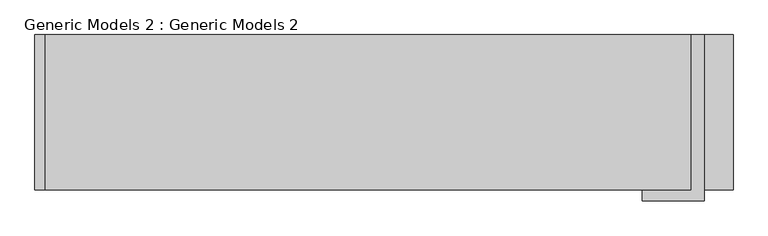
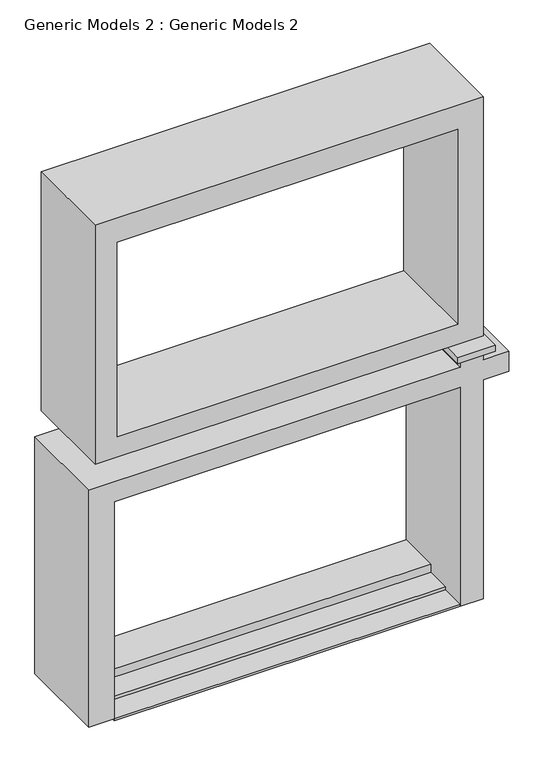
"""IFC4 building model written with IfcOpenShell, lengths in millimetres: proxy geometry, Generic Models 2 : Generic Models 2."""

from ifc_helpers import new_model, si_unit, frame, origin, place, context, project, spatial, polyline, outline, extrude, source, transform, mapped, element, save


def generic_models_2_generic_models_2_cc28d5f6(model_context):
    return source(origin(), model_context, "Body", "SweptSolid", [
        extrude(outline(polyline([(6400.8, -7427.5624893), (6400.8, -12113.8624893), (3352.8, -12113.8624893), (3352.8, -7427.5624893), (6400.8, -7427.5624893)]), holes=[polyline([(6096.0, -11847.1624893), (6096.0, -7739.1386409), (3611.0690813, -7739.1386409), (3611.0690813, -11847.1624893), (6096.0, -11847.1624893)])]), frame((0.0, -14113.1642742, 0.0), z_axis=(0.0, 1.0, 0.0), x_axis=(0.0, 0.0, 1.0)), (0.0, 0.0, 1.0), 1125.9602367),
        extrude(outline(polyline([(-7783.1624893, -12987.2040375), (-7330.8179528, -12987.2040375), (-7330.8179528, -14193.7040375), (-7783.1624893, -14193.7040375), (-7783.1624893, -12987.2040375)])), frame((0.0, 0.0, 3167.927738), z_axis=(0.0, 0.0, 1.0), x_axis=(1.0, 0.0, 0.0)), (0.0, 0.0, 1.0), 76.2),
        extrude(outline(polyline([(25.813216, -11885.2624893), (2792.6450587, -11885.2624893), (2792.6450587, -7709.0871232), (0.0, -7709.0871232), (0.0, -7427.5624893), (2792.6450587, -7427.5624893), (2792.6450587, -7121.9545456), (3048.0, -7121.9545456), (3048.0, -7427.5624893), (3167.927738, -7427.5624893), (3167.927738, -7709.0871232), (3048.0, -7709.0871232), (3048.0, -12190.0624893), (25.813216, -12190.0624893), (25.813216, -11885.2624893)])), frame((0.0, -14113.1642742, 0.0), z_axis=(0.0, 1.0, 0.0), x_axis=(0.0, 0.0, 1.0)), (0.0, 0.0, 1.0), 1125.9602367),
        extrude(outline(polyline([(-13808.3642742, 63.4172343), (-13503.5642742, 63.4172343), (-13503.5642742, 167.195182), (-12987.2040375, 167.195182), (-12987.2040375, 0.0), (-14113.1642742, 0.0), (-14113.1642742, 25.813216), (-13808.3642742, 25.813216), (-13808.3642742, 63.4172343)])), frame((-11885.2624893, 0.0, 0.0), z_axis=(1.0, 0.0, 0.0), x_axis=(0.0, 1.0, 0.0)), (0.0, 0.0, 1.0), 4176.1753662),
    ])


if __name__ == "__main__":
    model = new_model("IFC4")
    model_context = context("Model", 3, world=origin())
    ifc_project = project(units=[si_unit("LENGTHUNIT", "METRE", prefix="MILLI")], contexts=[model_context])
    site = spatial("IfcSite", under=ifc_project)
    building = spatial("IfcBuilding", under=site)
    placement = place(None, origin())
    generic_models_2_generic_models_2_shape = generic_models_2_generic_models_2_cc28d5f6(model_context)
    element("IfcBuildingElementProxy", 1, Name="Generic Models 2 : Generic Models 2", ObjectType="Generic Models 2 : Generic Models 2", at=placement, inside=building, context=model_context, shape_type="MappedRepresentation", body=[
        mapped(generic_models_2_generic_models_2_shape, transform((0.0, 0.0, 0.0), x_axis=(1.0, 0.0, 0.0), y_axis=(0.0, 1.0, 0.0), z_axis=(0.0, 0.0, 1.0))),
    ])
    save(model, "model.ifc")
